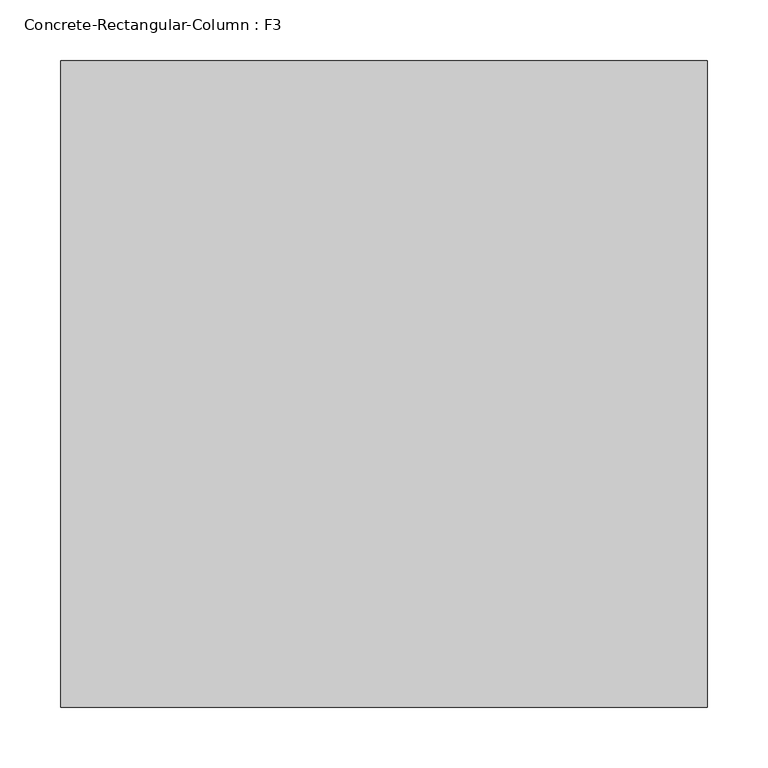
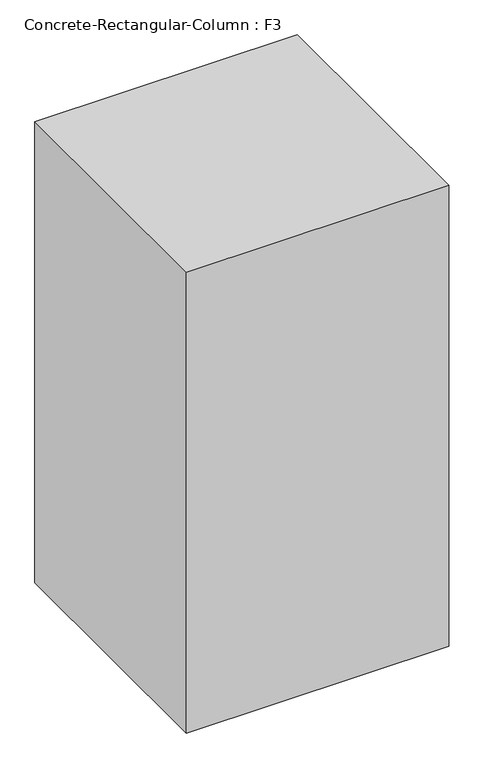
"""IFC4 building model written with IfcOpenShell, lengths in millimetres: column geometry, Concrete-Rectangular-Column : F3."""

from ifc_helpers import new_model, si_unit, origin, origin_with_axes, place, context, project, spatial, polyline, outline, extrude, source, transform, mapped, element, save


def concrete_rectangular_column_f3_aae16e16(model_context):
    return source(origin(), model_context, "Body", "SweptSolid", [
        extrude(outline(polyline([(266.7, 266.7), (266.7, -266.7), (-266.7, -266.7), (-266.7, 266.7), (266.7, 266.7)])), origin_with_axes(), (0.0, 0.0, 1.0), 990.6),
    ])


if __name__ == "__main__":
    model = new_model("IFC4")
    model_context = context("Model", 3, world=origin())
    ifc_project = project(units=[si_unit("LENGTHUNIT", "METRE", prefix="MILLI")], contexts=[model_context])
    site = spatial("IfcSite", under=ifc_project)
    building = spatial("IfcBuilding", under=site)
    placement = place(None, origin())
    concrete_rectangular_column_f3_shape = concrete_rectangular_column_f3_aae16e16(model_context)
    element("IfcColumn", 1, ObjectType="Concrete-Rectangular-Column : F3", at=placement, inside=building, context=model_context, shape_type="MappedRepresentation", body=[
        mapped(concrete_rectangular_column_f3_shape, transform((0.0, 0.0, 0.0), x_axis=(1.0, 0.0, 0.0), y_axis=(0.0, 1.0, 0.0), z_axis=(0.0, 0.0, 1.0))),
    ])
    save(model, "model.ifc")

# Revit data of these elements
# Type "Concrete-Rectangular-Column : F3"
#   b = 533.4 mm
#   h = 533.4 mm
#   Structural Material [instance default] = Concrete, Cast-in-Place gray
# Element 1 (IfcColumn, "Concrete-Rectangular-Column : F3")
#   Materials on its faces: "Concrete, Cast-in-Place gray"
# Materials
#   "Concrete, Cast-in-Place gray": class "Concrete", colour RGB 192 192 192, transparency 0, Description = "Cast-in-place concrete", Cost = 0
